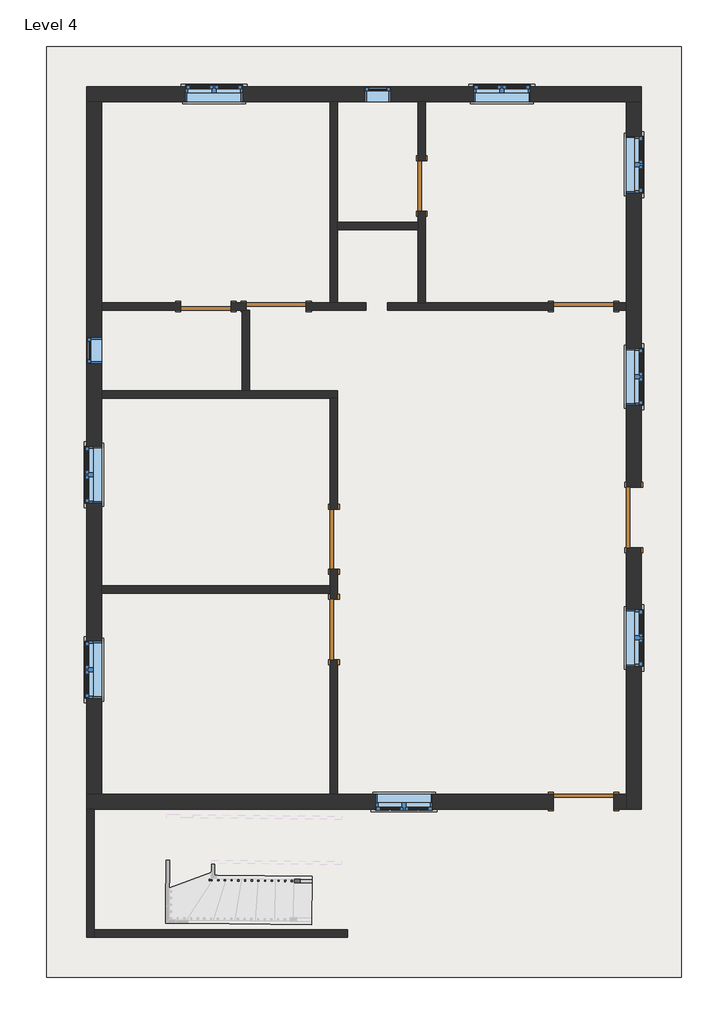
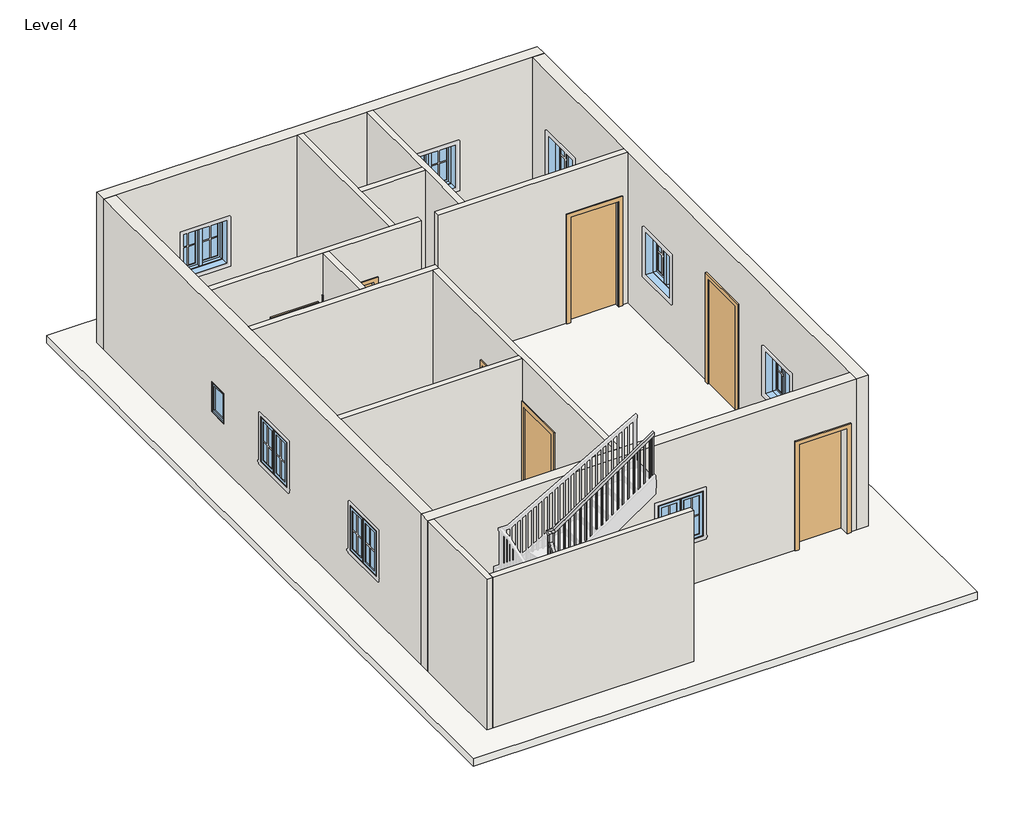
# One storey, part 1 of 2: 15 walls, 10 windows, 8 doors, 1 railing, 1 roof.
"""IFC4 building model written with IfcOpenShell, lengths in millimetres."""

from ifc_helpers import new_model, si_unit, frame, origin, place, context, project, spatial, polyline, outline, extrude, faceted_brep, transform, mapped, element, save
from components import door_f2b275c1, door_e5f9f3c4, door_305aa2a5, door_a90ba1ad, door_0ca8825f, window_aa618e30, window_339605e1

model = new_model("IFC4")

# Units and contexts
model_context = context("Model", 3, world=origin())
ifc_project = project(units=[si_unit("LENGTHUNIT", "METRE", prefix="MILLI")], contexts=[model_context])

# Site, building, storey
site = spatial("IfcSite", under=ifc_project)
building = spatial("IfcBuilding", under=site)
storey = spatial("IfcBuildingStorey", under=building, Name="Level 4", Elevation=6400.8)

# Doors
placement = place(None, origin())
door_shape = door_f2b275c1(model_context)
element("IfcDoor", 1, ObjectType="Single-Flush : 30\" x 80\"", at=placement, inside=storey, context=model_context, shape_type="MappedRepresentation", body=[
    mapped(door_shape, transform((-295.4747832, 5557.2532079, 6400.8), x_axis=(0.0, -1.0, 0.0), y_axis=(1.0, 0.0, 0.0), z_axis=(0.0, 0.0, 1.0))),
])
element("IfcDoor", 2, ObjectType="Single-Flush : 30\" x 80\"", at=placement, inside=storey, context=model_context, shape_type="MappedRepresentation", body=[
    mapped(door_shape, transform((-3572.0747832, 3728.4532079, 6400.8), x_axis=(1.0, 0.0, 0.0), y_axis=(0.0, 1.0, 0.0), z_axis=(0.0, 0.0, 1.0))),
])
door_2_shape = door_e5f9f3c4(model_context)
element("IfcDoor", 3, ObjectType="Single-Flush : 36\" x 84\"", at=placement, inside=storey, context=model_context, shape_type="MappedRepresentation", body=[
    mapped(door_2_shape, transform((-2505.2747832, 3728.4532079, 6400.8), x_axis=(1.0, 0.0, 0.0), y_axis=(0.0, 1.0, 0.0), z_axis=(0.0, 0.0, 1.0))),
])
element("IfcDoor", 4, ObjectType="Single-Flush : 36\" x 84\"", at=placement, inside=storey, context=model_context, shape_type="MappedRepresentation", body=[
    mapped(door_2_shape, transform((2161.9752168, 3728.4532079, 6400.8), x_axis=(1.0, 0.0, 0.0), y_axis=(0.0, 1.0, 0.0), z_axis=(0.0, 0.0, 1.0))),
])
element("IfcDoor", 5, ObjectType="Single-Flush : 36\" x 84\"", at=placement, inside=storey, context=model_context, shape_type="MappedRepresentation", body=[
    mapped(door_2_shape, transform((-1628.9747832, -1173.7467921, 6400.8), x_axis=(0.0, 1.0, 0.0), y_axis=(-1.0, 0.0, 0.0), z_axis=(0.0, 0.0, 1.0))),
])
door_3_shape = door_305aa2a5(model_context)
element("IfcDoor", 6, ObjectType="Single-Flush : 36\" x 84\"", at=placement, inside=storey, context=model_context, shape_type="MappedRepresentation", body=[
    mapped(door_3_shape, transform((-1628.9747832, 197.8532079, 6400.8), x_axis=(0.0, -1.0, 0.0), y_axis=(1.0, 0.0, 0.0), z_axis=(0.0, 0.0, 1.0))),
])
door_4_shape = door_a90ba1ad(model_context)
element("IfcDoor", 7, ObjectType="Single-Flush : 36\" x 84\"", at=placement, inside=storey, context=model_context, shape_type="MappedRepresentation", body=[
    mapped(door_4_shape, transform((2923.9752168, 528.0532079, 6400.8), x_axis=(0.0, -1.0, 0.0), y_axis=(1.0, 0.0, 0.0), z_axis=(0.0, 0.0, 1.0))),
])
door_5_shape = door_0ca8825f(model_context)
element("IfcDoor", 8, ObjectType="Single-Flush : 36\" x 84\"", at=placement, inside=storey, context=model_context, shape_type="MappedRepresentation", body=[
    mapped(door_5_shape, transform((2161.9752168, -3783.5967921, 6400.8), x_axis=(1.0, 0.0, 0.0), y_axis=(0.0, 1.0, 0.0), z_axis=(0.0, 0.0, 1.0))),
])

# Railing
element("IfcRailing", 9, ObjectType="Handrail - Rectangular", at=placement, inside=storey, context=model_context, shape_type="SolidModel", body=[
    faceted_brep([(-1962.1803506, -5016.2038017, 7484.5333333), (-1962.1803506, -5016.2038017, 7423.0793596), (-1961.6349602, -4965.4067295, 7423.0793596), (-1961.6349602, -4965.4067295, 7484.5333333), (-3413.6283866, -5000.6201116, 8472.6756169), (-3464.4254588, -5000.0747212, 8445.8041661), (-3463.8800684, -4949.2776489, 8445.8041661), (-3413.0829962, -4949.8230393, 8472.6756169), (-3413.6283866, -5000.6201116, 8689.761538), (-3464.4254588, -5000.0747212, 8638.961538), (-3463.8800684, -4949.2776489, 8638.961538), (-3413.0829962, -4949.8230393, 8689.761538), (-3540.6210672, -4999.2566356, 8689.761538), (-3540.6210672, -4999.2566356, 8638.961538), (-3489.2786045, -4949.0049537, 8638.961538), (-3489.2786045, -4949.0049537, 8689.761538), (-3539.2575912, -4872.2639549, 8689.761538), (-3538.9677931, -4845.272478, 8638.961538), (-3488.1707209, -4845.8178684, 8638.961538), (-3488.4605189, -4872.8093453, 8689.761538), (-3537.8941152, -4745.2712743, 8877.8249579), (-3537.3487248, -4694.4742021, 8862.2786564), (-3486.5516525, -4695.0195925, 8862.2786564), (-3487.0970429, -4745.8166647, 8877.8249579), (-3537.8941152, -4745.2712743, 9045.876961), (-3537.3487248, -4694.4742021, 8995.076961), (-3486.5516525, -4695.0195925, 8995.076961), (-3487.0970429, -4745.8166647, 9045.876961), (-3536.5306392, -4618.2785937, 9045.876961), (-3536.5306392, -4618.2785937, 8995.076961), (-3486.2789573, -4669.6210563, 8995.076961), (-3486.2789573, -4669.6210563, 9045.876961), (-3409.5379585, -4619.6420697, 9045.876961), (-3393.6525863, -4619.8126254, 8995.076961), (-3394.1979767, -4670.6096976, 8995.076961), (-3410.0833489, -4670.439142, 9045.876961), (-1509.4062983, -4640.0431191, 10363.2), (-1509.9516887, -4690.8401913, 10363.2), (-1509.9516887, -4690.8401913, 10301.3869912), (-1509.4062983, -4640.0431191, 10301.3869912)], [[[0, 1, 2, 3]], [[1, 0, 4, 5]], [[2, 1, 5, 6]], [[3, 2, 6, 7]], [[0, 3, 7, 4]], [[5, 4, 8, 9]], [[6, 5, 9, 10]], [[7, 6, 10, 11]], [[4, 7, 11, 8]], [[9, 8, 12, 13]], [[10, 9, 13, 14]], [[11, 10, 14, 15]], [[8, 11, 15, 12]], [[13, 12, 16, 17]], [[14, 13, 17, 18]], [[15, 14, 18, 19]], [[12, 15, 19, 16]], [[17, 16, 20, 21]], [[18, 17, 21, 22]], [[19, 18, 22, 23]], [[16, 19, 23, 20]], [[21, 20, 24, 25]], [[22, 21, 25, 26]], [[23, 22, 26, 27]], [[20, 23, 27, 24]], [[25, 24, 28, 29]], [[26, 25, 29, 30]], [[27, 26, 30, 31]], [[24, 27, 31, 28]], [[29, 28, 32, 33]], [[30, 29, 33, 34]], [[31, 30, 34, 35]], [[28, 31, 35, 32]], [[36, 37, 38, 39]], [[33, 32, 36, 39]], [[34, 33, 39, 38]], [[35, 34, 38, 37]], [[32, 35, 37, 36]]]),
    extrude(outline(polyline([(221.9968897, -19.05), (235.2031102, 0.0), (1200.994449, 0.0), (1200.994449, -19.05), (221.9968897, -19.05)])), frame((-1590.7427644, -4674.0968508, 10480.4611157), z_axis=(0.01073603161956521, 0.9999423671517594, 0.0), x_axis=(0.0, 0.0, -1.0)), (0.0, 0.0, 1.0), 19.05),
    extrude(outline(polyline([(221.9968898, -19.05), (235.2031102, 0.0), (1130.5612733, 0.0), (1130.5612733, -19.05), (221.9968898, -19.05)])), frame((-1692.3369089, -4673.00607, 10410.02794), z_axis=(0.01073603161956521, 0.9999423671517594, 0.0), x_axis=(0.0, 0.0, -1.0)), (0.0, 0.0, 1.0), 19.05),
    extrude(outline(polyline([(221.9968897, -19.05), (235.2031102, 0.0), (1060.1280975, 0.0), (1060.1280975, -19.05), (221.9968897, -19.05)])), frame((-1793.9310534, -4671.9152892, 10339.5947642), z_axis=(0.01073603161956521, 0.9999423671517594, 0.0), x_axis=(0.0, 0.0, -1.0)), (0.0, 0.0, 1.0), 19.05),
    extrude(outline(polyline([(221.9968898, -19.05), (235.2031103, 0.0), (1159.0282552, 0.0), (1159.0282552, -19.05), (221.9968898, -19.05)])), frame((-1895.5251979, -4670.8245084, 10269.1615885), z_axis=(0.01073603161956521, 0.9999423671517594, 0.0), x_axis=(0.0, 0.0, -1.0)), (0.0, 0.0, 1.0), 19.05),
    extrude(outline(polyline([(221.9968898, -19.05), (235.2031102, 0.0), (1088.5950794, 0.0), (1088.5950794, -19.05), (221.9968898, -19.05)])), frame((-1997.1193424, -4669.7337275, 10198.7284127), z_axis=(0.01073603161956521, 0.9999423671517594, 0.0), x_axis=(0.0, 0.0, -1.0)), (0.0, 0.0, 1.0), 19.05),
    extrude(outline(polyline([(221.9968898, -19.05), (235.2031103, 0.0), (1187.495237, 0.0), (1187.495237, -19.05), (221.9968898, -19.05)])), frame((-2098.7134869, -4668.6429467, 10128.295237), z_axis=(0.01073603161956521, 0.9999423671517594, 0.0), x_axis=(0.0, 0.0, -1.0)), (0.0, 0.0, 1.0), 19.05),
    extrude(outline(polyline([(221.9968898, -19.05), (235.2031102, 0.0), (1117.0620612, 0.0), (1117.0620612, -19.05), (221.9968898, -19.05)])), frame((-2200.3076314, -4667.5521659, 10057.8620612), z_axis=(0.01073603161956521, 0.9999423671517594, 0.0), x_axis=(0.0, 0.0, -1.0)), (0.0, 0.0, 1.0), 19.05),
    extrude(outline(polyline([(221.9968897, -19.0499999), (235.2031102, 0.0), (1046.6288854, 0.0), (1046.6288854, -19.0499999), (221.9968897, -19.0499999)])), frame((-2301.9017759, -4666.4613851, 9987.4288854), z_axis=(0.01073603161956521, 0.9999423671517594, 0.0), x_axis=(0.0, 0.0, -1.0)), (0.0, 0.0, 1.0), 19.05),
    extrude(outline(polyline([(221.9968898, -19.0499999), (235.2031102, 0.0), (1145.529043, 0.0), (1145.529043, -19.0499999), (221.9968898, -19.0499999)])), frame((-2403.4959204, -4665.3706043, 9916.9957097), z_axis=(0.01073603161956521, 0.9999423671517594, 0.0), x_axis=(0.0, 0.0, -1.0)), (0.0, 0.0, 1.0), 19.05),
    extrude(outline(polyline([(221.9968897, -19.05), (235.2031102, 0.0), (1075.0958672, 0.0), (1075.0958672, -19.05), (221.9968897, -19.05)])), frame((-2505.090065, -4664.2798235, 9846.5625339), z_axis=(0.01073603161956521, 0.9999423671517594, 0.0), x_axis=(0.0, 0.0, -1.0)), (0.0, 0.0, 1.0), 19.05),
    extrude(outline(polyline([(221.9968898, -19.05), (235.2031103, 0.0), (1004.6626915, 0.0), (1004.6626915, -19.05), (221.9968898, -19.05)])), frame((-2606.6842095, -4663.1890427, 9776.1293582), z_axis=(0.01073603161956521, 0.9999423671517594, 0.0), x_axis=(0.0, 0.0, -1.0)), (0.0, 0.0, 1.0), 19.05),
    extrude(outline(polyline([(221.9968898, -19.05), (235.2031102, 0.0), (1103.5628491, 0.0), (1103.5628491, -19.05), (221.9968898, -19.05)])), frame((-2708.278354, -4662.0982619, 9705.6961824), z_axis=(0.01073603161956521, 0.9999423671517594, 0.0), x_axis=(0.0, 0.0, -1.0)), (0.0, 0.0, 1.0), 19.05),
    extrude(outline(polyline([(221.9968898, -19.05), (235.2031103, 0.0), (1033.1296734, 0.0), (1033.1296734, -19.05), (221.9968898, -19.05)])), frame((-2809.8724985, -4661.007481, 9635.2630067), z_axis=(0.01073603161956521, 0.9999423671517594, 0.0), x_axis=(0.0, 0.0, -1.0)), (0.0, 0.0, 1.0), 19.05),
    extrude(outline(polyline([(221.9968898, -19.05), (235.2031102, 0.0), (1132.0298309, 0.0), (1132.0298309, -19.05), (221.9968898, -19.05)])), frame((-2911.466643, -4659.9167002, 9564.8298309), z_axis=(0.01073603161956521, 0.9999423671517594, 0.0), x_axis=(0.0, 0.0, -1.0)), (0.0, 0.0, 1.0), 19.05),
    extrude(outline(polyline([(221.9968897, -19.05), (235.2031102, 0.0), (1061.5966551, 0.0), (1061.5966551, -19.05), (221.9968897, -19.05)])), frame((-3013.0607875, -4658.8259194, 9494.3966551), z_axis=(0.01073603161956521, 0.9999423671517594, 0.0), x_axis=(0.0, 0.0, -1.0)), (0.0, 0.0, 1.0), 19.05),
    extrude(outline(polyline([(221.9968898, -19.05), (235.2031102, 0.0), (991.1634794, 0.0), (991.1634794, -19.05), (221.9968898, -19.05)])), frame((-3114.654932, -4657.7351386, 9423.9634794), z_axis=(0.01073603161956521, 0.9999423671517594, 0.0), x_axis=(0.0, 0.0, -1.0)), (0.0, 0.0, 1.0), 19.05),
    extrude(outline(polyline([(221.9968897, -19.05), (235.2031102, 0.0), (1090.0636369, 0.0), (1090.0636369, -19.05), (221.9968897, -19.05)])), frame((-3216.2490765, -4656.6443578, 9353.5303036), z_axis=(0.01073603161956521, 0.9999423671517594, 0.0), x_axis=(0.0, 0.0, -1.0)), (0.0, 0.0, 1.0), 19.05),
    extrude(outline(polyline([(221.9968898, -19.05), (235.2031103, 0.0), (1019.6304612, 0.0), (1019.6304612, -19.05), (221.9968898, -19.05)])), frame((-3317.843221, -4655.553577, 9283.0971279), z_axis=(0.01073603161956521, 0.9999423671517594, 0.0), x_axis=(0.0, 0.0, -1.0)), (0.0, 0.0, 1.0), 19.05),
    extrude(outline(polyline([(221.9968898, -19.05), (235.2031102, 0.0), (1118.5306188, 0.0), (1118.5306188, -19.05), (221.9968898, -19.05)])), frame((-3419.4373655, -4654.4627962, 9212.6639521), z_axis=(0.01073603161956521, 0.9999423671517594, 0.0), x_axis=(0.0, 0.0, -1.0)), (0.0, 0.0, 1.0), 19.05),
    extrude(outline(polyline([(-3502.2553031, -4678.9750729), (-3521.3042052, -4678.7705515), (-3521.0996838, -4659.7216494), (-3502.0507817, -4659.9261708), (-3502.2553031, -4678.9750729)])), frame((0.0, 0.0, 7924.8), z_axis=(0.0, 0.0, 1.0), x_axis=(1.0, 0.0, 0.0)), (0.0, 0.0, 1.0), 1070.276961),
    extrude(outline(polyline([(214.4952435, -19.05), (242.7047565, 0.0), (1222.5739377, 0.0), (1222.5739377, -19.05), (214.4952435, -19.05)])), frame((-3503.3460839, -4780.5692174, 8978.0406044), z_axis=(-0.9999423671517594, 0.010736031619565895, 0.0), x_axis=(0.0, 0.0, -1.0)), (0.0, 0.0, 1.0), 19.05),
    extrude(outline(polyline([(214.4952435, -19.05), (242.7047565, 0.0), (1072.1232018, 0.0), (1072.1232018, -19.05), (214.4952435, -19.05)])), frame((-3504.4368647, -4882.1633619, 8827.5898685), z_axis=(-0.9999423671517594, 0.010736031619565895, 0.0), x_axis=(0.0, 0.0, -1.0)), (0.0, 0.0, 1.0), 19.05),
    extrude(outline(polyline([(-3476.1931112, -4965.0213631), (-3476.3976326, -4984.0702652), (-3495.4465347, -4983.8657438), (-3495.2420133, -4964.8168417), (-3476.1931112, -4965.0213631)])), frame((0.0, 0.0, 7586.1333333), z_axis=(0.0, 0.0, 1.0), x_axis=(1.0, 0.0, 0.0)), (0.0, 0.0, 1.0), 1052.8282047),
    extrude(outline(polyline([(235.0842231, -19.05), (222.115777, 0.0), (1203.1900014, 0.0), (1203.1900014, -19.05), (235.0842231, -19.05)])), frame((-3393.8523902, -4984.9565246, 8619.9900014), z_axis=(0.01073603161956537, 0.9999423671517593, 0.0), x_axis=(0.0, 0.0, -1.0)), (0.0, 0.0, 1.0), 19.05),
    extrude(outline(polyline([(235.084223, -19.05), (222.1157769, 0.0), (1134.0249555, 0.0), (1134.0249555, -19.05), (235.084223, -19.05)])), frame((-3292.2582457, -4986.0473054, 8550.8249555), z_axis=(0.01073603161956537, 0.9999423671517593, 0.0), x_axis=(0.0, 0.0, -1.0)), (0.0, 0.0, 1.0), 19.05),
    extrude(outline(polyline([(235.0842231, -19.05), (222.115777, 0.0), (1234.193243, 0.0), (1234.193243, -19.05), (235.0842231, -19.05)])), frame((-3190.6641012, -4987.1380862, 8481.6599097), z_axis=(0.01073603161956537, 0.9999423671517593, 0.0), x_axis=(0.0, 0.0, -1.0)), (0.0, 0.0, 1.0), 19.05),
    extrude(outline(polyline([(235.084223, -19.05), (222.1157769, 0.0), (1165.0281971, 0.0), (1165.0281971, -19.05), (235.084223, -19.05)])), frame((-3089.0699567, -4988.228867, 8412.4948638), z_axis=(0.01073603161956537, 0.9999423671517593, 0.0), x_axis=(0.0, 0.0, -1.0)), (0.0, 0.0, 1.0), 19.05),
    extrude(outline(polyline([(235.084223, -19.05), (222.1157769, 0.0), (1265.1964847, 0.0), (1265.1964847, -19.05), (235.084223, -19.05)])), frame((-2987.4758122, -4989.3196478, 8343.329818), z_axis=(0.01073603161956537, 0.9999423671517593, 0.0), x_axis=(0.0, 0.0, -1.0)), (0.0, 0.0, 1.0), 19.05),
    extrude(outline(polyline([(235.0842231, -19.05), (222.115777, 0.0), (1196.0314389, 0.0), (1196.0314389, -19.05), (235.0842231, -19.05)])), frame((-2885.8816677, -4990.4104286, 8274.1647722), z_axis=(0.01073603161956537, 0.9999423671517593, 0.0), x_axis=(0.0, 0.0, -1.0)), (0.0, 0.0, 1.0), 19.05),
    extrude(outline(polyline([(235.084223, -19.05), (222.1157769, 0.0), (1296.1997263, 0.0), (1296.1997263, -19.05), (235.084223, -19.05)])), frame((-2784.2875232, -4991.5012094, 8204.9997263), z_axis=(0.01073603161956537, 0.9999423671517593, 0.0), x_axis=(0.0, 0.0, -1.0)), (0.0, 0.0, 1.0), 19.05),
    extrude(outline(polyline([(235.0842231, -19.05), (222.115777, 0.0), (1227.0346805, 0.0), (1227.0346805, -19.05), (235.0842231, -19.05)])), frame((-2682.6933787, -4992.5919903, 8135.8346805), z_axis=(0.01073603161956537, 0.9999423671517593, 0.0), x_axis=(0.0, 0.0, -1.0)), (0.0, 0.0, 1.0), 19.05),
    extrude(outline(polyline([(235.084223, -19.05), (222.1157769, 0.0), (1157.8696346, 0.0), (1157.8696346, -19.05), (235.084223, -19.05)])), frame((-2581.0992342, -4993.6827711, 8066.6696346), z_axis=(0.01073603161956537, 0.9999423671517593, 0.0), x_axis=(0.0, 0.0, -1.0)), (0.0, 0.0, 1.0), 19.05),
    extrude(outline(polyline([(235.0842231, -19.05), (222.115777, 0.0), (1258.0379221, 0.0), (1258.0379221, -19.05), (235.0842231, -19.05)])), frame((-2479.5050897, -4994.7735519, 7997.5045888), z_axis=(0.01073603161956537, 0.9999423671517593, 0.0), x_axis=(0.0, 0.0, -1.0)), (0.0, 0.0, 1.0), 19.05),
    extrude(outline(polyline([(235.084223, -19.05), (222.1157769, 0.0), (1188.8728762, 0.0), (1188.8728762, -19.05), (235.084223, -19.05)])), frame((-2377.9109452, -4995.8643327, 7928.3395429), z_axis=(0.01073603161956537, 0.9999423671517593, 0.0), x_axis=(0.0, 0.0, -1.0)), (0.0, 0.0, 1.0), 19.05),
    extrude(outline(polyline([(235.084223, -19.05), (222.115777, 0.0), (1119.7078304, 0.0), (1119.7078304, -19.05), (235.084223, -19.05)])), frame((-2276.3168007, -4996.9551135, 7859.1744971), z_axis=(0.01073603161956537, 0.9999423671517593, 0.0), x_axis=(0.0, 0.0, -1.0)), (0.0, 0.0, 1.0), 19.05),
    extrude(outline(polyline([(235.0842231, -19.05), (222.115777, 0.0), (1219.876118, 0.0), (1219.876118, -19.05), (235.0842231, -19.05)])), frame((-2174.7226562, -4998.0458943, 7790.0094513), z_axis=(0.01073603161956537, 0.9999423671517593, 0.0), x_axis=(0.0, 0.0, -1.0)), (0.0, 0.0, 1.0), 19.05),
    extrude(outline(polyline([(235.084223, -19.05), (222.1157769, 0.0), (1150.7110721, 0.0), (1150.7110721, -19.05), (235.084223, -19.05)])), frame((-2073.1285117, -4999.1366751, 7720.8444054), z_axis=(0.01073603161956537, 0.9999423671517593, 0.0), x_axis=(0.0, 0.0, -1.0)), (0.0, 0.0, 1.0), 19.05),
    extrude(outline(polyline([(-3501.9826079, -4653.5765368), (-3521.03151, -4653.3720154), (-3520.8269886, -4634.3231133), (-3501.7780865, -4634.5276347), (-3501.9826079, -4653.5765368)])), frame((0.0, 0.0, 7924.8), z_axis=(0.0, 0.0, 1.0), x_axis=(1.0, 0.0, 0.0)), (0.0, 0.0, 1.0), 1070.276961),
    extrude(outline(polyline([(-3505.3231241, -4964.7086043), (-3505.5276455, -4983.7575064), (-3524.5765476, -4983.552985), (-3524.3720262, -4964.5040829), (-3505.3231241, -4964.7086043)])), frame((0.0, 0.0, 7586.1333333), z_axis=(0.0, 0.0, 1.0), x_axis=(1.0, 0.0, 0.0)), (0.0, 0.0, 1.0), 1052.8282047),
    extrude(outline(polyline([(221.9968897, -19.05), (235.2031102, 0.0), (1243.9172142, 0.0), (1243.9172142, -19.05), (221.9968897, -19.05)])), frame((-1528.8301563, -4674.7615848, 10523.3838809), z_axis=(0.01073603161956521, 0.9999423671517594, 0.0), x_axis=(0.0, 0.0, -1.0)), (0.0, 0.0, 1.0), 19.05),
    extrude(outline(polyline([(235.084223, -19.05), (222.1157769, 0.0), (1088.0302493, 0.0), (1088.0302493, -19.05), (235.084223, -19.05)])), frame((-1981.0588182, -5000.1251952, 7658.1635826), z_axis=(0.01073603161956537, 0.9999423671517593, 0.0), x_axis=(0.0, 0.0, -1.0)), (0.0, 0.0, 1.0), 19.05),
])

# Roof
element("IfcRoof", 10, ObjectType="Generic - 12\"", at=placement, inside=storey, context=model_context, shape_type="SweptSolid", body=[
    extrude(outline(polyline([(-5991.4247832, 7671.8032079), (3647.8752168, 7671.8032079), (3647.8752168, -6450.5967921), (-5991.4247832, -6450.5967921), (-5991.4247832, 7671.8032079)])), frame((0.0, 0.0, 6248.4), z_axis=(0.0, 0.0, 1.0), x_axis=(1.0, 0.0, 0.0)), (0.0, 0.0, 1.0), 152.4),
])

# Walls
element("IfcWall", 11, ObjectType="WALL4.5\"", at=placement, inside=storey, context=model_context, shape_type="Brep", body=[
    faceted_brep([(-2048.0747832, 3671.3032079, 8534.4), (-2048.0747832, 3671.3032079, 6400.8), (-1141.0287494, 3671.3032079, 6400.8), (-1141.0287494, 3671.3032079, 9448.8), (-2905.3247832, 3671.3032079, 9448.8), (-3019.6247832, 3671.3032079, 9448.8), (-5153.2247832, 3671.3032079, 9448.8), (-5153.2247832, 3671.3032079, 6400.8), (-3953.0747832, 3671.3032079, 6400.8), (-3953.0747832, 3671.3032079, 8432.8), (-3191.0747832, 3671.3032079, 8432.8), (-3191.0747832, 3671.3032079, 6400.8), (-3019.6247832, 3671.3032079, 6400.8), (-2962.4747832, 3671.3032079, 6400.8), (-2962.4747832, 3671.3032079, 8534.4), (-1141.0287494, 3785.6032079, 6400.8), (-1571.8247832, 3785.6032079, 6400.8), (-1686.1247832, 3785.6032079, 6400.8), (-2048.0747832, 3785.6032079, 6400.8), (-2048.0747832, 3785.6032079, 8534.4), (-2962.4747832, 3785.6032079, 8534.4), (-2962.4747832, 3785.6032079, 6400.8), (-3191.0747832, 3785.6032079, 6400.8), (-3191.0747832, 3785.6032079, 8432.8), (-3953.0747832, 3785.6032079, 8432.8), (-3953.0747832, 3785.6032079, 6400.8), (-5153.2247832, 3785.6032079, 6400.8), (-5153.2247832, 3785.6032079, 9448.8), (-1686.1247832, 3785.6032079, 9448.8), (-1571.8247832, 3785.6032079, 9448.8), (-1141.0287494, 3785.6032079, 9448.8)], [[[0, 1, 2, 3, 4, 5, 6, 7, 8, 9, 10, 11, 12, 13, 14]], [[15, 16, 17, 18, 19, 20, 21, 22, 23, 24, 25, 26, 27, 28, 29, 30]], [[8, 7, 26, 25]], [[2, 1, 18, 17, 16, 15]], [[13, 12, 11, 22, 21]], [[3, 2, 15, 30]], [[7, 6, 27, 26]], [[23, 22, 11, 10]], [[24, 23, 10, 9]], [[25, 24, 9, 8]], [[19, 18, 1, 0]], [[20, 19, 0, 14]], [[21, 20, 14, 13]], [[6, 5, 4, 3, 30, 29, 28, 27]]]),
])
element("IfcWall", 12, ObjectType="WALL4.5\"", at=placement, inside=storey, context=model_context, shape_type="Brep", body=[
    faceted_brep([(2619.1752168, 3671.3032079, 8534.4), (2619.1752168, 3671.3032079, 6400.8), (2809.6752168, 3671.3032079, 6400.8), (2809.6752168, 3671.3032079, 9448.8), (-812.7163761, 3671.3032079, 9448.8), (-812.7163761, 3671.3032079, 6400.8), (1704.7752168, 3671.3032079, 6400.8), (1704.7752168, 3671.3032079, 8534.4), (2809.6752168, 3785.6032079, 6400.8), (2619.1752168, 3785.6032079, 6400.8), (2619.1752168, 3785.6032079, 8534.4), (1704.7752168, 3785.6032079, 8534.4), (1704.7752168, 3785.6032079, 6400.8), (-238.3247832, 3785.6032079, 6400.8), (-352.6247832, 3785.6032079, 6400.8), (-812.7163761, 3785.6032079, 6400.8), (-812.7163761, 3785.6032079, 9448.8), (-352.6247832, 3785.6032079, 9448.8), (-238.3247832, 3785.6032079, 9448.8), (2809.6752168, 3785.6032079, 9448.8)], [[[0, 1, 2, 3, 4, 5, 6, 7]], [[8, 9, 10, 11, 12, 13, 14, 15, 16, 17, 18, 19]], [[6, 5, 15, 14, 13, 12]], [[2, 1, 9, 8]], [[5, 4, 16, 15]], [[3, 2, 8, 19]], [[10, 9, 1, 0]], [[11, 10, 0, 7]], [[12, 11, 7, 6]], [[4, 3, 19, 18, 17, 16]]]),
])
element("IfcWall", 13, ObjectType="WALL4.5\"", at=placement, inside=storey, context=model_context, shape_type="Brep", body=[
    faceted_brep([(-1686.1247832, 6833.6032079, 6400.8), (-1686.1247832, 3785.6032079, 6400.8), (-1686.1247832, 3785.6032079, 9448.8), (-1686.1247832, 6833.6032079, 9448.8), (-1571.8247832, 6833.6032079, 6400.8), (-1571.8247832, 6833.6032079, 9448.8), (-1571.8247832, 5004.8032079, 9448.8), (-1571.8247832, 4890.5032079, 9448.8), (-1571.8247832, 3785.6032079, 9448.8), (-1571.8247832, 3785.6032079, 6400.8), (-1571.8247832, 4890.5032079, 6400.8), (-1571.8247832, 5004.8032079, 6400.8)], [[[0, 1, 2, 3]], [[4, 5, 6, 7, 8, 9, 10, 11]], [[1, 0, 4, 11, 10, 9]], [[0, 3, 5, 4]], [[2, 1, 9, 8]], [[3, 2, 8, 7, 6, 5]]]),
])
element("IfcWall", 14, ObjectType="WALL4.5\"", at=placement, inside=storey, context=model_context, shape_type="SweptSolid", body=[
    extrude(outline(polyline([(-352.6247832, 4890.5032079), (-1571.8247832, 4890.5032079), (-1571.8247832, 5004.8032079), (-352.6247832, 5004.8032079), (-352.6247832, 4890.5032079)])), frame((0.0, 0.0, 6400.8), z_axis=(0.0, 0.0, 1.0), x_axis=(1.0, 0.0, 0.0)), (0.0, 0.0, 1.0), 3048.0),
])
element("IfcWall", 15, ObjectType="WALL4.5\"", at=placement, inside=storey, context=model_context, shape_type="Brep", body=[
    faceted_brep([(-352.6247832, 5176.2532079, 8432.8), (-352.6247832, 5176.2532079, 6400.8), (-352.6247832, 5004.8032079, 6400.8), (-352.6247832, 4890.5032079, 6400.8), (-352.6247832, 3785.6032079, 6400.8), (-352.6247832, 3785.6032079, 9448.8), (-352.6247832, 4890.5032079, 9448.8), (-352.6247832, 5004.8032079, 9448.8), (-352.6247832, 6833.6032079, 9448.8), (-352.6247832, 6833.6032079, 6400.8), (-352.6247832, 5938.2532079, 6400.8), (-352.6247832, 5938.2532079, 8432.8), (-238.3247832, 3785.6032079, 6400.8), (-238.3247832, 5176.2532079, 6400.8), (-238.3247832, 5176.2532079, 8432.8), (-238.3247832, 5938.2532079, 8432.8), (-238.3247832, 5938.2532079, 6400.8), (-238.3247832, 6833.6032079, 6400.8), (-238.3247832, 6833.6032079, 9448.8), (-238.3247832, 3785.6032079, 9448.8)], [[[0, 1, 2, 3, 4, 5, 6, 7, 8, 9, 10, 11]], [[12, 13, 14, 15, 16, 17, 18, 19]], [[10, 9, 17, 16]], [[4, 3, 2, 1, 13, 12]], [[9, 8, 18, 17]], [[5, 4, 12, 19]], [[14, 13, 1, 0]], [[15, 14, 0, 11]], [[16, 15, 11, 10]], [[8, 7, 6, 5, 19, 18]]]),
])
element("IfcWall", 16, ObjectType="WALL4.5\"", at=placement, inside=storey, context=model_context, shape_type="Brep", body=[
    faceted_brep([(-3019.6247832, 3671.3032079, 6400.8), (-3019.6247832, 2452.1032079, 6400.8), (-3019.6247832, 2452.1032079, 9448.8), (-3019.6247832, 3671.3032079, 9448.8), (-2905.3247832, 3671.3032079, 6400.8), (-2905.3247832, 3671.3032079, 9448.8), (-2905.3247832, 2452.1032079, 9448.8), (-2905.3247832, 2452.1032079, 6400.8), (-2962.4747832, 3671.3032079, 6400.8)], [[[0, 1, 2, 3]], [[4, 5, 6, 7]], [[1, 0, 8, 4, 7]], [[0, 3, 5, 4, 8]], [[2, 1, 7, 6]], [[3, 2, 6, 5]]]),
])
element("IfcWall", 17, ObjectType="WALL4.5\"", at=placement, inside=storey, context=model_context, shape_type="Brep", body=[
    faceted_brep([(-5153.2247832, 2337.8032079, 6400.8), (-1686.1247832, 2337.8032079, 6400.8), (-1571.8247832, 2337.8032079, 6400.8), (-1571.8247832, 2337.8032079, 9448.8), (-1686.1247832, 2337.8032079, 9448.8), (-5153.2247832, 2337.8032079, 9448.8), (-5153.2247832, 2452.1032079, 6400.8), (-5153.2247832, 2452.1032079, 9448.8), (-3019.6247832, 2452.1032079, 9448.8), (-2905.3247832, 2452.1032079, 9448.8), (-1571.8247832, 2452.1032079, 9448.8), (-1571.8247832, 2452.1032079, 6400.8), (-2905.3247832, 2452.1032079, 6400.8), (-3019.6247832, 2452.1032079, 6400.8)], [[[0, 1, 2, 3, 4, 5]], [[6, 7, 8, 9, 10, 11, 12, 13]], [[2, 1, 0, 6, 13, 12, 11]], [[0, 5, 7, 6]], [[3, 2, 11, 10]], [[5, 4, 3, 10, 9, 8, 7]]]),
])
element("IfcWall", 18, ObjectType="WALL4.5\"", at=placement, inside=storey, context=model_context, shape_type="Brep", body=[
    faceted_brep([(-1686.1247832, -259.3467921, 6400.8), (-1686.1247832, -506.9967921, 6400.8), (-1686.1247832, -621.2967921, 6400.8), (-1686.1247832, -716.5467921, 6400.8), (-1686.1247832, -716.5467921, 8534.4), (-1686.1247832, -1630.9467921, 8534.4), (-1686.1247832, -1630.9467921, 6400.8), (-1686.1247832, -3669.2967921, 6400.8), (-1686.1247832, -3669.2967921, 9448.8), (-1686.1247832, -621.2967921, 9448.8), (-1686.1247832, -506.9967921, 9448.8), (-1686.1247832, 2337.8032079, 9448.8), (-1686.1247832, 2337.8032079, 6400.8), (-1686.1247832, 655.0532079, 6400.8), (-1686.1247832, 655.0532079, 8534.4), (-1686.1247832, -259.3467921, 8534.4), (-1571.8247832, -716.5467921, 8534.4), (-1571.8247832, -716.5467921, 6400.8), (-1571.8247832, -259.3467921, 6400.8), (-1571.8247832, -259.3467921, 8534.4), (-1571.8247832, 655.0532079, 8534.4), (-1571.8247832, 655.0532079, 6400.8), (-1571.8247832, 2337.8032079, 6400.8), (-1571.8247832, 2337.8032079, 9448.8), (-1571.8247832, -3669.2967921, 9448.8), (-1571.8247832, -3669.2967921, 6400.8), (-1571.8247832, -1630.9467921, 6400.8), (-1571.8247832, -1630.9467921, 8534.4)], [[[0, 1, 2, 3, 4, 5, 6, 7, 8, 9, 10, 11, 12, 13, 14, 15]], [[16, 17, 18, 19, 20, 21, 22, 23, 24, 25, 26, 27]], [[13, 12, 22, 21]], [[26, 25, 7, 6]], [[18, 17, 3, 2, 1, 0]], [[12, 11, 23, 22]], [[8, 7, 25, 24]], [[19, 18, 0, 15]], [[20, 19, 15, 14]], [[21, 20, 14, 13]], [[4, 3, 17, 16]], [[5, 4, 16, 27]], [[6, 5, 27, 26]], [[11, 10, 9, 8, 24, 23]]]),
])
element("IfcWall", 19, ObjectType="WALL4.5\"", at=placement, inside=storey, context=model_context, shape_type="SweptSolid", body=[
    extrude(outline(polyline([(-1686.1247832, -621.2967921), (-5153.2247832, -621.2967921), (-5153.2247832, -506.9967921), (-1686.1247832, -506.9967921), (-1686.1247832, -621.2967921)])), frame((0.0, 0.0, 6400.8), z_axis=(0.0, 0.0, 1.0), x_axis=(1.0, 0.0, 0.0)), (0.0, 0.0, 1.0), 3048.0),
])
element("IfcWall", 20, ObjectType="WALL4.5\"", at=placement, inside=storey, context=model_context, shape_type="Brep", body=[
    faceted_brep([(-5381.8247832, -3897.8967921, 6400.8), (-5381.8247832, -5840.9967921, 6400.8), (-5381.8247832, -5840.9967921, 9448.8), (-5381.8247832, -3897.8967921, 9448.8), (-5267.5247832, -3897.8967921, 6400.8), (-5267.5247832, -3897.8967921, 9448.8), (-5267.5247832, -5726.6967921, 9448.8), (-5267.5247832, -5840.9967921, 9448.8), (-5267.5247832, -5840.9967921, 6400.8), (-5267.5247832, -5726.6967921, 6400.8)], [[[0, 1, 2, 3]], [[4, 5, 6, 7, 8, 9]], [[1, 0, 4, 9, 8]], [[0, 3, 5, 4]], [[2, 1, 8, 7]], [[3, 2, 7, 6, 5]]]),
])
element("IfcWall", 21, ObjectType="WALL4.5\"", at=placement, inside=storey, context=model_context, shape_type="SweptSolid", body=[
    extrude(outline(polyline([(-1419.4247832, -5840.9967921), (-5267.5247832, -5840.9967921), (-5267.5247832, -5726.6967921), (-1419.4247832, -5726.6967921), (-1419.4247832, -5840.9967921)])), frame((0.0, 0.0, 6400.8), z_axis=(0.0, 0.0, 1.0), x_axis=(1.0, 0.0, 0.0)), (0.0, 0.0, 1.0), 3048.0),
])
element("IfcWall", 22, ObjectType="WALL9\"", at=placement, inside=storey, context=model_context, shape_type="Brep", body=[
    faceted_brep([(-5381.8247832, 6833.6032079, 6400.8), (-5153.2247832, 6833.6032079, 6400.8), (-1686.1247832, 6833.6032079, 6400.8), (-1571.8247832, 6833.6032079, 6400.8), (-352.6247832, 6833.6032079, 6400.8), (-238.3247832, 6833.6032079, 6400.8), (2809.6752168, 6833.6032079, 6400.8), (3038.2752168, 6833.6032079, 6400.8), (3038.2752168, 6833.6032079, 9448.8), (2809.6752168, 6833.6032079, 9448.8), (-238.3247832, 6833.6032079, 9448.8), (-352.6247832, 6833.6032079, 9448.8), (-1571.8247832, 6833.6032079, 9448.8), (-1686.1247832, 6833.6032079, 9448.8), (-5153.2247832, 6833.6032079, 9448.8), (-5381.8247832, 6833.6032079, 9448.8), (-759.0247832, 6833.6032079, 7924.8), (-759.0247832, 6833.6032079, 7315.2), (-1165.4247832, 6833.6032079, 7315.2), (-1165.4247832, 6833.6032079, 7924.8), (-3016.4497832, 6833.6032079, 8229.6), (-3016.4497832, 6833.6032079, 7315.2), (-3880.0497832, 6833.6032079, 7315.2), (-3880.0497832, 6833.6032079, 8229.6), (1355.5252168, 6833.6032079, 8229.6), (1355.5252168, 6833.6032079, 7315.2), (491.9252168, 6833.6032079, 7315.2), (491.9252168, 6833.6032079, 8229.6), (-5381.8247832, 7062.2032079, 6400.8), (-5381.8247832, 7062.2032079, 9448.8), (3038.2752168, 7062.2032079, 9448.8), (3038.2752168, 7062.2032079, 6400.8), (-759.0247832, 7062.2032079, 7924.8), (-1165.4247832, 7062.2032079, 7924.8), (-1165.4247832, 7062.2032079, 7315.2), (-759.0247832, 7062.2032079, 7315.2), (-3016.4497832, 7062.2032079, 8229.6), (-3880.0497832, 7062.2032079, 8229.6), (-3880.0497832, 7062.2032079, 7315.2), (-3016.4497832, 7062.2032079, 7315.2), (1355.5252168, 7062.2032079, 8229.6), (491.9252168, 7062.2032079, 8229.6), (491.9252168, 7062.2032079, 7315.2), (1355.5252168, 7062.2032079, 7315.2)], [[[0, 1, 2, 3, 4, 5, 6, 7, 8, 9, 10, 11, 12, 13, 14, 15], [16, 17, 18, 19], [20, 21, 22, 23], [24, 25, 26, 27]], [[28, 29, 30, 31], [32, 33, 34, 35], [36, 37, 38, 39], [40, 41, 42, 43]], [[7, 6, 5, 4, 3, 2, 1, 0, 28, 31]], [[8, 7, 31, 30]], [[0, 15, 29, 28]], [[17, 16, 32, 35]], [[18, 17, 35, 34]], [[19, 18, 34, 33]], [[16, 19, 33, 32]], [[21, 20, 36, 39]], [[22, 21, 39, 38]], [[23, 22, 38, 37]], [[20, 23, 37, 36]], [[25, 24, 40, 43]], [[26, 25, 43, 42]], [[27, 26, 42, 41]], [[24, 27, 41, 40]], [[15, 14, 13, 12, 11, 10, 9, 8, 30, 29]]]),
])
element("IfcWall", 23, ObjectType="WALL9\"", at=placement, inside=storey, context=model_context, shape_type="Brep", body=[
    faceted_brep([(2809.6752168, 70.8532079, 8534.4), (2809.6752168, 70.8532079, 6400.8), (2809.6752168, -3669.2967921, 6400.8), (2809.6752168, -3897.8967921, 6400.8), (2809.6752168, -3897.8967921, 9448.8), (2809.6752168, -3669.2967921, 9448.8), (2809.6752168, 3671.3032079, 9448.8), (2809.6752168, 3785.6032079, 9448.8), (2809.6752168, 6833.6032079, 9448.8), (2809.6752168, 6833.6032079, 6400.8), (2809.6752168, 3785.6032079, 6400.8), (2809.6752168, 3671.3032079, 6400.8), (2809.6752168, 985.2532079, 6400.8), (2809.6752168, 985.2532079, 8534.4), (2809.6752168, 5449.3032079, 8229.6), (2809.6752168, 5449.3032079, 7315.2), (2809.6752168, 6312.9032079, 7315.2), (2809.6752168, 6312.9032079, 8229.6), (2809.6752168, 2229.8532079, 8229.6), (2809.6752168, 2229.8532079, 7315.2), (2809.6752168, 3093.4532079, 7315.2), (2809.6752168, 3093.4532079, 8229.6), (2809.6752168, -1732.5467921, 8229.6), (2809.6752168, -1732.5467921, 7315.2), (2809.6752168, -868.9467921, 7315.2), (2809.6752168, -868.9467921, 8229.6), (3038.2752168, -3897.8967921, 6400.8), (3038.2752168, 70.8532079, 6400.8), (3038.2752168, 70.8532079, 8534.4), (3038.2752168, 985.2532079, 8534.4), (3038.2752168, 985.2532079, 6400.8), (3038.2752168, 6833.6032079, 6400.8), (3038.2752168, 6833.6032079, 9448.8), (3038.2752168, -3897.8967921, 9448.8), (3038.2752168, 5449.3032079, 8229.6), (3038.2752168, 6312.9032079, 8229.6), (3038.2752168, 6312.9032079, 7315.2), (3038.2752168, 5449.3032079, 7315.2), (3038.2752168, 2229.8532079, 8229.6), (3038.2752168, 3093.4532079, 8229.6), (3038.2752168, 3093.4532079, 7315.2), (3038.2752168, 2229.8532079, 7315.2), (3038.2752168, -1732.5467921, 8229.6), (3038.2752168, -868.9467921, 8229.6), (3038.2752168, -868.9467921, 7315.2), (3038.2752168, -1732.5467921, 7315.2)], [[[0, 1, 2, 3, 4, 5, 6, 7, 8, 9, 10, 11, 12, 13], [14, 15, 16, 17], [18, 19, 20, 21], [22, 23, 24, 25]], [[26, 27, 28, 29, 30, 31, 32, 33], [34, 35, 36, 37], [38, 39, 40, 41], [42, 43, 44, 45]], [[3, 2, 1, 27, 26]], [[12, 11, 10, 9, 31, 30]], [[9, 8, 32, 31]], [[4, 3, 26, 33]], [[28, 27, 1, 0]], [[29, 28, 0, 13]], [[30, 29, 13, 12]], [[15, 14, 34, 37]], [[16, 15, 37, 36]], [[17, 16, 36, 35]], [[14, 17, 35, 34]], [[19, 18, 38, 41]], [[20, 19, 41, 40]], [[21, 20, 40, 39]], [[18, 21, 39, 38]], [[23, 22, 42, 45]], [[24, 23, 45, 44]], [[25, 24, 44, 43]], [[22, 25, 43, 42]], [[8, 7, 6, 5, 4, 33, 32]]]),
])
element("IfcWall", 24, ObjectType="WALL9\"", at=placement, inside=storey, context=model_context, shape_type="Brep", body=[
    faceted_brep([(2809.6752168, -3669.2967921, 6400.8), (2619.1752168, -3669.2967921, 6400.8), (2619.1752168, -3669.2967921, 8534.4), (1704.7752168, -3669.2967921, 8534.4), (1704.7752168, -3669.2967921, 6400.8), (-1571.8247832, -3669.2967921, 6400.8), (-1686.1247832, -3669.2967921, 6400.8), (-5153.2247832, -3669.2967921, 6400.8), (-5381.8247832, -3669.2967921, 6400.8), (-5381.8247832, -3669.2967921, 9448.8), (-5153.2247832, -3669.2967921, 9448.8), (-1686.1247832, -3669.2967921, 9448.8), (-1571.8247832, -3669.2967921, 9448.8), (2809.6752168, -3669.2967921, 9448.8), (-993.9747832, -3669.2967921, 8229.6), (-993.9747832, -3669.2967921, 7315.2), (-130.3747832, -3669.2967921, 7315.2), (-130.3747832, -3669.2967921, 8229.6), (2619.1752168, -3897.8967921, 8534.4), (2619.1752168, -3897.8967921, 6400.8), (2809.6752168, -3897.8967921, 6400.8), (2809.6752168, -3897.8967921, 9448.8), (-5267.5247832, -3897.8967921, 9448.8), (-5381.8247832, -3897.8967921, 9448.8), (-5381.8247832, -3897.8967921, 6400.8), (-5267.5247832, -3897.8967921, 6400.8), (1704.7752168, -3897.8967921, 6400.8), (1704.7752168, -3897.8967921, 8534.4), (-993.9747832, -3897.8967921, 8229.6), (-130.3747832, -3897.8967921, 8229.6), (-130.3747832, -3897.8967921, 7315.2), (-993.9747832, -3897.8967921, 7315.2)], [[[0, 1, 2, 3, 4, 5, 6, 7, 8, 9, 10, 11, 12, 13], [14, 15, 16, 17]], [[18, 19, 20, 21, 22, 23, 24, 25, 26, 27], [28, 29, 30, 31]], [[20, 19, 1, 0]], [[26, 25, 24, 8, 7, 6, 5, 4]], [[0, 13, 21, 20]], [[9, 8, 24, 23]], [[2, 1, 19, 18]], [[3, 2, 18, 27]], [[4, 3, 27, 26]], [[15, 14, 28, 31]], [[16, 15, 31, 30]], [[17, 16, 30, 29]], [[14, 17, 29, 28]], [[13, 12, 11, 10, 9, 23, 22, 21]]]),
])
element("IfcWall", 25, ObjectType="WALL9\"", at=placement, inside=storey, context=model_context, shape_type="Brep", body=[
    faceted_brep([(-5153.2247832, -3669.2967921, 6400.8), (-5153.2247832, -621.2967921, 6400.8), (-5153.2247832, -506.9967921, 6400.8), (-5153.2247832, 2337.8032079, 6400.8), (-5153.2247832, 2452.1032079, 6400.8), (-5153.2247832, 3671.3032079, 6400.8), (-5153.2247832, 3785.6032079, 6400.8), (-5153.2247832, 6833.6032079, 6400.8), (-5153.2247832, 6833.6032079, 9448.8), (-5153.2247832, 3785.6032079, 9448.8), (-5153.2247832, 3671.3032079, 9448.8), (-5153.2247832, 2452.1032079, 9448.8), (-5153.2247832, 2337.8032079, 9448.8), (-5153.2247832, -506.9967921, 9448.8), (-5153.2247832, -621.2967921, 9448.8), (-5153.2247832, -3669.2967921, 9448.8), (-5153.2247832, 3264.9032079, 7924.8), (-5153.2247832, 3264.9032079, 7315.2), (-5153.2247832, 2858.5032079, 7315.2), (-5153.2247832, 2858.5032079, 7924.8), (-5153.2247832, 1607.5532079, 8229.6), (-5153.2247832, 1607.5532079, 7315.2), (-5153.2247832, 743.9532079, 7315.2), (-5153.2247832, 743.9532079, 8229.6), (-5153.2247832, -1351.5467921, 8229.6), (-5153.2247832, -1351.5467921, 7315.2), (-5153.2247832, -2215.1467921, 7315.2), (-5153.2247832, -2215.1467921, 8229.6), (-5381.8247832, -3669.2967921, 6400.8), (-5381.8247832, -3669.2967921, 9448.8), (-5381.8247832, 6833.6032079, 9448.8), (-5381.8247832, 6833.6032079, 6400.8), (-5381.8247832, 3264.9032079, 7924.8), (-5381.8247832, 2858.5032079, 7924.8), (-5381.8247832, 2858.5032079, 7315.2), (-5381.8247832, 3264.9032079, 7315.2), (-5381.8247832, 1607.5532079, 8229.6), (-5381.8247832, 743.9532079, 8229.6), (-5381.8247832, 743.9532079, 7315.2), (-5381.8247832, 1607.5532079, 7315.2), (-5381.8247832, -1351.5467921, 8229.6), (-5381.8247832, -2215.1467921, 8229.6), (-5381.8247832, -2215.1467921, 7315.2), (-5381.8247832, -1351.5467921, 7315.2)], [[[0, 1, 2, 3, 4, 5, 6, 7, 8, 9, 10, 11, 12, 13, 14, 15], [16, 17, 18, 19], [20, 21, 22, 23], [24, 25, 26, 27]], [[28, 29, 30, 31], [32, 33, 34, 35], [36, 37, 38, 39], [40, 41, 42, 43]], [[7, 6, 5, 4, 3, 2, 1, 0, 28, 31]], [[8, 7, 31, 30]], [[0, 15, 29, 28]], [[17, 16, 32, 35]], [[18, 17, 35, 34]], [[19, 18, 34, 33]], [[16, 19, 33, 32]], [[21, 20, 36, 39]], [[22, 21, 39, 38]], [[23, 22, 38, 37]], [[20, 23, 37, 36]], [[25, 24, 40, 43]], [[26, 25, 43, 42]], [[27, 26, 42, 41]], [[24, 27, 41, 40]], [[15, 14, 13, 12, 11, 10, 9, 8, 30, 29]]]),
])

# Windows
window_shape = window_aa618e30(model_context)
element("IfcWindow", 26, ObjectType="Fixed : 16\" x 24\"", at=placement, inside=storey, context=model_context, shape_type="MappedRepresentation", body=[
    mapped(window_shape, transform((-924.1247832, 6947.9032079, 6400.8), x_axis=(1.0, 0.0, 0.0), y_axis=(0.0, 1.0, 0.0), z_axis=(0.0, 0.0, 1.0))),
])
element("IfcWindow", 27, ObjectType="Fixed : 16\" x 24\"", at=placement, inside=storey, context=model_context, shape_type="MappedRepresentation", body=[
    mapped(window_shape, transform((-5267.5247832, 3099.8032079, 6400.8), x_axis=(0.0, 1.0, 0.0), y_axis=(-1.0, 0.0, 0.0), z_axis=(0.0, 0.0, 1.0))),
])
window_2_shape = window_339605e1(model_context)
element("IfcWindow", 28, ObjectType="Window-Casement-Double : 34\" x 36\"", at=placement, inside=storey, context=model_context, shape_type="MappedRepresentation", body=[
    mapped(window_2_shape, transform((-3448.2497832, 6947.9032079, 6400.8), x_axis=(1.0, 0.0, 0.0), y_axis=(0.0, 1.0, 0.0), z_axis=(0.0, 0.0, 1.0))),
])
element("IfcWindow", 29, ObjectType="Window-Casement-Double : 34\" x 36\"", at=placement, inside=storey, context=model_context, shape_type="MappedRepresentation", body=[
    mapped(window_2_shape, transform((923.7252168, 6947.9032079, 6400.8), x_axis=(1.0, 0.0, 0.0), y_axis=(0.0, 1.0, 0.0), z_axis=(0.0, 0.0, 1.0))),
])
element("IfcWindow", 30, ObjectType="Window-Casement-Double : 34\" x 36\"", at=placement, inside=storey, context=model_context, shape_type="MappedRepresentation", body=[
    mapped(window_2_shape, transform((2923.9752168, 5881.1032079, 6400.8), x_axis=(0.0, -1.0, 0.0), y_axis=(1.0, 0.0, 0.0), z_axis=(0.0, 0.0, 1.0))),
])
element("IfcWindow", 31, ObjectType="Window-Casement-Double : 34\" x 36\"", at=placement, inside=storey, context=model_context, shape_type="MappedRepresentation", body=[
    mapped(window_2_shape, transform((2923.9752168, 2661.6532079, 6400.8), x_axis=(0.0, -1.0, 0.0), y_axis=(1.0, 0.0, 0.0), z_axis=(0.0, 0.0, 1.0))),
])
element("IfcWindow", 32, ObjectType="Window-Casement-Double : 34\" x 36\"", at=placement, inside=storey, context=model_context, shape_type="MappedRepresentation", body=[
    mapped(window_2_shape, transform((2923.9752168, -1300.7467921, 6400.8), x_axis=(0.0, -1.0, 0.0), y_axis=(1.0, 0.0, 0.0), z_axis=(0.0, 0.0, 1.0))),
])
element("IfcWindow", 33, ObjectType="Window-Casement-Double : 34\" x 36\"", at=placement, inside=storey, context=model_context, shape_type="MappedRepresentation", body=[
    mapped(window_2_shape, transform((-5267.5247832, 1175.7532079, 6400.8), x_axis=(0.0, 1.0, 0.0), y_axis=(-1.0, 0.0, 0.0), z_axis=(0.0, 0.0, 1.0))),
])
element("IfcWindow", 34, ObjectType="Window-Casement-Double : 34\" x 36\"", at=placement, inside=storey, context=model_context, shape_type="MappedRepresentation", body=[
    mapped(window_2_shape, transform((-5267.5247832, -1783.3467921, 6400.8), x_axis=(0.0, 1.0, 0.0), y_axis=(-1.0, 0.0, 0.0), z_axis=(0.0, 0.0, 1.0))),
])
element("IfcWindow", 35, ObjectType="Window-Casement-Double : 34\" x 36\"", at=placement, inside=storey, context=model_context, shape_type="MappedRepresentation", body=[
    mapped(window_2_shape, transform((-562.1747832, -3783.5967921, 6400.8), x_axis=(-1.0, 0.0, 0.0), y_axis=(0.0, -1.0, 0.0), z_axis=(0.0, 0.0, 1.0))),
])

save(model, "model.ifc")

# Revit data of these elements
# Type "Single-Flush : 30\" x 80\""
#   Type Mark = "5"
#   Construction Type Id = "MDOOR"
#   Assembly Code = "C1020"
#   Analytic Construction = "Metal"
#   Thickness = 0' - 2"
#   Heat Transfer Coefficient (U) = 0.651978 BTU/(h·ft²·°F)
#   Height = 6' - 8"
#   Trim Projection Ext = 0' - 1"
#   Trim Projection Int = 0' - 1"
#   Trim Width = 0' - 3"
#   Width = 2' - 6"
#   Define Thermal Properties by = 1
#   Define Thermal Properties by = 1
#   Door Material = Door - Panel
#   Frame Material = Door - Frame
#   Visual Light Transmittance = 0
#   Solar Heat Gain Coefficient = 0
#   Function = (empty or 0)
#   Wall Closure = (empty or 0)
# Type "Single-Flush : 36\" x 84\""
#   Type Mark = "1"
#   Construction Type Id = "MDOOR"
#   Assembly Code = "C1020"
#   Analytic Construction = "Metal"
#   Thickness = 0' - 2"
#   Heat Transfer Coefficient (U) = 0.651978 BTU/(h·ft²·°F)
#   Height = 7' - 0"
#   Trim Projection Ext = 0' - 1"
#   Trim Projection Int = 0' - 1"
#   Trim Width = 0' - 3"
#   Width = 3' - 0"
#   Define Thermal Properties by = 1
#   Define Thermal Properties by = 1
#   Door Material = Door - Panel
#   Frame Material = Door - Frame
#   Visual Light Transmittance = 0
#   Solar Heat Gain Coefficient = 0
#   Function = (empty or 0)
#   Wall Closure = (empty or 0)
# Type "Handrail - Rectangular"
#   Assembly Code = "C2010400"
#   built-in parameter 1008612 = 0.0416667 (stored number, unit not read)
#   built-in parameter 1008611 = 0.0416667 (stored number, unit not read)
#   built-in parameter 1008609 = 0.333333 (stored number, unit not read)
#   built-in parameter 1008604 = 0.166667 (stored number, unit not read)
#   built-in parameter 1008603 = 0.166667 (stored number, unit not read)
#   Railing Height = 3' - 0"
#   built-in parameter 1008630 = 2
#   built-in parameter 1008610 = 2
#   built-in parameter 1008618 = Baluster - Square : 3/4"
# Type "Generic - 12\""
#   Assembly Code = "B1020"
#   Layers, outside or top first: 0' - 6" no material (function 1)
# Type "WALL4.5\""
#   Assembly Code = "B2010"
#   Layers, outside or top first: 0' - 4 1/2" no material (function 1)
# Type "WALL9\""
#   Assembly Code = "B2010"
#   Layers, outside or top first: 0' - 9" no material (function 1)
# Type "Fixed : 16\" x 24\""
#   Type Mark = "4"
#   Construction Type Id = "GSP4R"
#   Assembly Code = "B2020100"
#   Analytic Construction = "1/8 in Pilkington single glazing"
#   Visual Light Transmittance = 0.9
#   Solar Heat Gain Coefficient = 0.78
#   Heat Transfer Coefficient (U) = 0.6496 BTU/(h·ft²·°F)
#   Height = 2' - 0"
#   Default Sill Height = 3' - 0"
#   Width = 1' - 4"
#   Window Inset = 0' - 0 3/4"
#   Define Thermal Properties by = 1
#   Define Thermal Properties by = 1
#   Glass Pane Material = Glass
#   Sash Material = Sash
#   Wall Closure = (empty or 0)
# Type "Window-Casement-Double : 34\" x 36\""
#   Type Mark = "14"
#   Fire Rating = "0.5h"
#   Assembly Code = "B2020100"
#   Analytic Construction = "Double glazing - domestic"
#   Frame Extension [instance default] = 0' - 0 1/4"
#   Window Inset [instance default] = 0' - 0"
#   Wall Thickness [instance default] = 0' - 6"
#   Interior Wall Closure [instance default] = 0' - 2 1/4"
#   Half Width = 1' - 5"
#   Visual Light Transmittance = 0.81
#   Thermal Resistance (R) = 1.8146 (h·ft²·°F)/BTU
#   Solar Heat Gain Coefficient = 0.76
#   Rough Width = 2' - 10 1/2"
#   Rough Height = 3' - 0 1/2"
#   Height = 3' - 0"
#   Heat Transfer Coefficient (U) = 0.5511 BTU/(h·ft²·°F)
#   Exterior Wall Closure [instance default] = 0' - 1 1/4"
#   Extension Jamb [instance default] = 0' - 2 1/4"
#   Default Sill Height = 3' - 0"
#   Width = 2' - 10"
#   Define Thermal Properties by = 0
#   Muntin Visibility = yes
#   Interior Trim Visibility [instance default] = yes
#   Exterior Trim Visibility [instance default] = yes
#   Extension Jamb Visibility [instance default] = yes
#   Interior Trim Material = Wood - Stained
#   Muntin Pattern = Muntin Pattern_2x2 : Muntin Pattern_2x2
#   Interior Trim = Trim-Window-Interior-Flat : Picture Frame
#   Interior Frame Material = Wood - Stained
#   Glass Panel Material = Glass
#   Exterior Trim Material = Clad - White
#   Exterior Trim = Trim-Window-Exterior-Flat : with Sill
#   Exterior Frame Material = Clad - White
#   Wall Closure = (empty or 0)
# Elements 1, 2 (IfcDoor, "Single-Flush : 30\" x 80\"")
#   Phase Created = New Construction
#   Materials on its faces: "Door - Frame", "Door - Panel"
# Elements 3, 4, 5, 6, 7, 8 (IfcDoor, "Single-Flush : 36\" x 84\"")
#   Phase Created = New Construction
#   Materials on its faces: "Door - Frame", "Door - Panel"
# Element 9 (IfcRailing, "Handrail - Rectangular")
#   Phase Created = New Construction
# Element 10 (IfcRoof, "Generic - 12\"")
#   built-in parameter 1001705 = 21 (stored number, unit not read)
#   built-in parameter 1001701 = -0.5 (stored number, unit not read)
#   built-in parameter 1001710 = 33615
#   Phase Created = New Construction
#   Materials on its faces: "Default Roof", "Carpet (1)"
# Elements 11, 12, 13, 14, 15, 16, 17, 18, 19 (IfcWall, "WALL4.5\"")
#   Top Offset = 0' - 0"
#   Base Offset = 0' - 0"
#   Unconnected Height = 10' - 0"
#   wall height = 10' - 0"
#   Phase Created = New Construction
#   Base Constraint = Level 4
#   Materials on its faces: "Default Wall"
# Elements 20, 21 (IfcWall, "WALL4.5\"")
#   Top Offset = 0' - 0"
#   Base Offset = 0' - 0"
#   Unconnected Height = 10' - 0"
#   wall height = 10' - 0"
#   Phase Created = New Construction
#   Base Constraint = Level 4
#   Materials on its faces: "Default Wall", "Carpet (1)"
# Elements 22, 23, 24, 25 (IfcWall, "WALL9\"")
#   Top Offset = 0' - 0"
#   Base Offset = 0' - 0"
#   Unconnected Height = 10' - 0"
#   wall height = 10' - 0"
#   Phase Created = New Construction
#   Base Constraint = Level 4
#   Materials on its faces: "Default Wall", "Carpet (1)"
# Element 26 (IfcWindow, "Fixed : 16\" x 24\"")
#   Mark = "21"
#   Phase Created = New Construction
#   Materials on its faces: "Sash", "Glass"
# Element 27 (IfcWindow, "Fixed : 16\" x 24\"")
#   Mark = "22"
#   Phase Created = New Construction
#   Materials on its faces: "Sash", "Glass"
# Element 28 (IfcWindow, "Window-Casement-Double : 34\" x 36\"")
#   Mark = "23"
#   Window Inset = 0' - 0"
#   Interior Wall Closure = 0' - 2 1/4"
#   Frame Extension = 0' - 0 1/4"
#   Exterior Wall Closure = 0' - 1 1/4"
#   Interior Trim Visibility = yes
#   Exterior Trim Visibility = yes
#   Phase Created = New Construction
#   Materials on its faces: "Wood - Stained", "Glass", "Clad - White"
# Element 29 (IfcWindow, "Window-Casement-Double : 34\" x 36\"")
#   Mark = "24"
#   Window Inset = 0' - 0"
#   Interior Wall Closure = 0' - 2 1/4"
#   Frame Extension = 0' - 0 1/4"
#   Exterior Wall Closure = 0' - 1 1/4"
#   Interior Trim Visibility = yes
#   Exterior Trim Visibility = yes
#   Phase Created = New Construction
#   Materials on its faces: "Wood - Stained", "Glass", "Clad - White"
# Element 30 (IfcWindow, "Window-Casement-Double : 34\" x 36\"")
#   Mark = "25"
#   Window Inset = 0' - 0"
#   Interior Wall Closure = 0' - 2 1/4"
#   Frame Extension = 0' - 0 1/4"
#   Exterior Wall Closure = 0' - 1 1/4"
#   Interior Trim Visibility = yes
#   Exterior Trim Visibility = yes
#   Phase Created = New Construction
#   Materials on its faces: "Wood - Stained", "Glass", "Clad - White"
# Element 31 (IfcWindow, "Window-Casement-Double : 34\" x 36\"")
#   Mark = "26"
#   Window Inset = 0' - 0"
#   Interior Wall Closure = 0' - 2 1/4"
#   Frame Extension = 0' - 0 1/4"
#   Exterior Wall Closure = 0' - 1 1/4"
#   Interior Trim Visibility = yes
#   Exterior Trim Visibility = yes
#   Phase Created = New Construction
#   Materials on its faces: "Wood - Stained", "Glass", "Clad - White"
# Element 32 (IfcWindow, "Window-Casement-Double : 34\" x 36\"")
#   Mark = "27"
#   Window Inset = 0' - 0"
#   Interior Wall Closure = 0' - 2 1/4"
#   Frame Extension = 0' - 0 1/4"
#   Exterior Wall Closure = 0' - 1 1/4"
#   Interior Trim Visibility = yes
#   Exterior Trim Visibility = yes
#   Phase Created = New Construction
#   Materials on its faces: "Wood - Stained", "Glass", "Clad - White"
# Element 33 (IfcWindow, "Window-Casement-Double : 34\" x 36\"")
#   Mark = "28"
#   Window Inset = 0' - 0"
#   Interior Wall Closure = 0' - 2 1/4"
#   Frame Extension = 0' - 0 1/4"
#   Exterior Wall Closure = 0' - 1 1/4"
#   Interior Trim Visibility = yes
#   Exterior Trim Visibility = yes
#   Phase Created = New Construction
#   Materials on its faces: "Wood - Stained", "Glass", "Clad - White"
# Element 34 (IfcWindow, "Window-Casement-Double : 34\" x 36\"")
#   Mark = "29"
#   Window Inset = 0' - 0"
#   Interior Wall Closure = 0' - 2 1/4"
#   Frame Extension = 0' - 0 1/4"
#   Exterior Wall Closure = 0' - 1 1/4"
#   Interior Trim Visibility = yes
#   Exterior Trim Visibility = yes
#   Phase Created = New Construction
#   Materials on its faces: "Wood - Stained", "Glass", "Clad - White"
# Element 35 (IfcWindow, "Window-Casement-Double : 34\" x 36\"")
#   Mark = "30"
#   Window Inset = 0' - 0"
#   Interior Wall Closure = 0' - 2 1/4"
#   Frame Extension = 0' - 0 1/4"
#   Exterior Wall Closure = 0' - 1 1/4"
#   Interior Trim Visibility = yes
#   Exterior Trim Visibility = yes
#   Phase Created = New Construction
#   Materials on its faces: "Wood - Stained", "Glass", "Clad - White"
# Materials
#   "Door - Panel": class "Wood", colour RGB 210 159 95, transparency 0, Cost = 0
#   "Door - Frame": colour RGB 118 70 51, transparency 0, Cost = 0
#   "Glass": class "Glass", colour RGB 0 128 192, transparency 0.75, Description = "Soda Lime Glass", Cost = 0
#   "Sash": class "Wood", colour RGB 224 178 126, transparency 0, Cost = 0
#   "Wood - Stained": class "Wood", colour RGB 224 178 126, transparency 0, Cost = 0
#   "Clad - White": class "Wood", colour RGB 242 242 238, transparency 0, Cost = 0
#   "Default Roof": colour RGB 88 101 114, transparency 0, Cost = 0
#   "Carpet (1)": class "Carpet", colour RGB 124 80 67, transparency 0, Description = "Interior finish", Cost = 0
#   "Default Wall": colour RGB 128 128 128, transparency 0, Cost = 0
